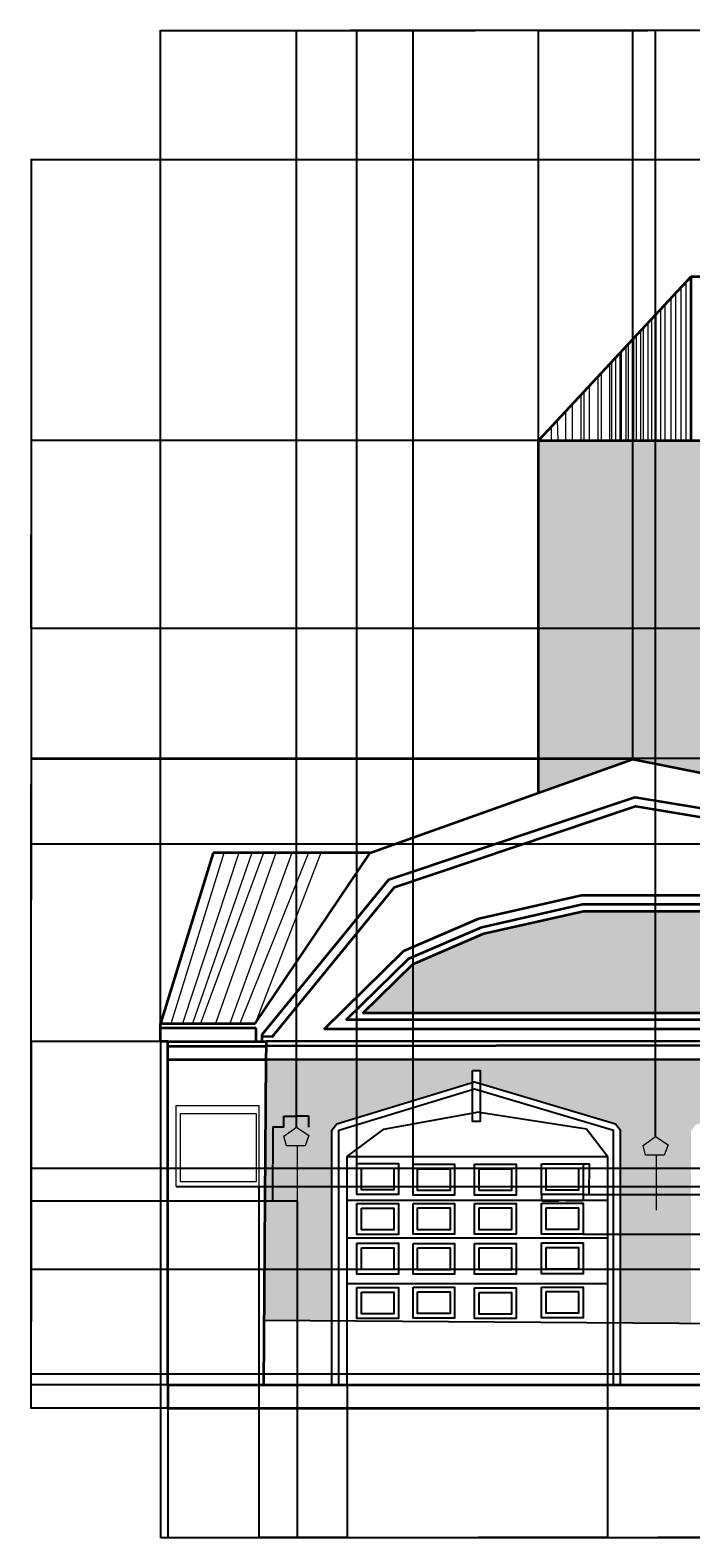
# Model space of a CAD drawing. Units: inches. Extents: x -46 to 1209, y 110 to 778.
# Tile 1 of 5: x -46 to 247, y 110 to 778. Entities that reach past the tile are written whole.
import ezdxf

# ---------------------------------------------------------------- set-up
doc = ezdxf.new("R2010")
doc.units = ezdxf.units.IN
doc.header["$MEASUREMENT"] = 0
for name, color, linetype, lineweight in [('A-ANNO-DIMS', 2, 'Continuous', 18), ('A-DOOR', 3, 'Continuous', 25), ('A-ELEV-BASE', 7, 'Continuous', 35), ('A-GLAZ', 4, 'Continuous', 20), ('A-ROOF', 7, 'Continuous', 35), ('A-ROOF-PATT', 8, 'Continuous', 13), ('A-WALL', 7, 'Continuous', 35), ('A-WALL-PATT', 252, 'Continuous', 13), ('A-WALL-TRIM', 42, 'Continuous', 25), ('E-LITE', 2, 'Continuous', 18)]:
    doc.layers.add(name, color=color, linetype=linetype, lineweight=lineweight)
doc.styles.get("Standard").update_dxf_attribs({"font": 'arial.ttf'})
doc.dimstyles.get("Standard").update_dxf_attribs({"dimtxt": 0.18, "dimasz": 0.18, "dimexe": 0.18, "dimexo": 0.0625, "dimgap": 0.09, "dimtad": 0, "dimtih": 1, "dimtoh": 1, "dimdec": 4, "dimzin": 0, "dimdsep": 46, "dimtxsty": 'Standard', "dimcen": 0.09, "dimadec": 0, "dimazin": 0, "dimtfac": 1, "dimtdec": 4, "dimtofl": 0, "dimtmove": 0, "dimatfit": 3, "dimfxl": 1, "dimtolj": 1, "dimtzin": 0, "dimarcsym": 0})

# ---------------------------------------------------------------- blocks, each defined once
blk = doc.blocks.new('WIN-SMALL-FRAME')
for points in [[(0, 35.97), (36.6, 35.97), (36.6, 0), (0, 0)], [(1.9, 32.4), (35.37, 32.4), (35.37, 2.05), (1.9, 2.05)]]:
    blk.add_lwpolyline(points, close=True)
blk = doc.blocks.new('PANEL-GARAGE-RAISED')
for points in [[(0, 13.64), (18.32, 13.64), (18.32, 0), (0, 0)], [(2, 11.64), (16.32, 11.64), (16.32, 2), (2, 2)]]:
    blk.add_lwpolyline(points, close=True)
blk = doc.blocks.new('KEYSTONE-GARAGE')
blk.add_lwpolyline([(0, 22.61), (3.38, 22.61), (3.38, 0), (0, 0)], close=True)
blk = doc.blocks.new('LIGHT-EXT-GARAGE')
blk.add_line((5.84, 24.47), (5.84, 0))
blk.add_lwpolyline([(5.84, 24.47), (1.13, 24.47), (0, 28.75), (5.52, 32.71), (11.04, 29.03), (9.34, 24.47), (5.84, 24.47)])
blk = doc.blocks.new('*D10')
at = {"layer": 'A-ANNO-DIMS', "color": 0, "lineweight": -2, "transparency": 16777216}
for p, q in [((180.55, 261.88), (180.55, 259.01)), ((198.86, 261.88), (198.86, 259.01)), ((180.73, 259.19), (188.16, 259.19)), ((198.68, 259.19), (191.25, 259.19))]:
    blk.add_line(p, q, dxfattribs=at)
at = {"layer": 'A-ANNO-DIMS', "color": 0, "transparency": 16777216}
for points in [[(180.73, 259.22), (180.73, 259.16), (180.55, 259.19)], [(198.68, 259.22), (198.68, 259.16), (198.86, 259.19)]]:
    blk.add_solid(points, dxfattribs=at)
at = {"layer": 'Defpoints', "color": 0, "transparency": 16777216}
for p in [(180.55, 261.94), (198.86, 261.94), (198.86, 259.19)]:
    blk.add_point(p, dxfattribs=at)
at = {"layer": 'A-ANNO-DIMS', "color": 0, "transparency": 16777216, "insert": (189.71, 259.19), "char_height": 0.18, "attachment_point": 5}
blk.add_mtext('\\A1;GARAGE PANEL 18 TYP.', dxfattribs=at)
blk = doc.blocks.new('*D11')
at = {"layer": 'A-ANNO-DIMS', "color": 0, "lineweight": -2, "transparency": 16777216}
for p, q in [((198.93, 275.58), (201.79, 275.58)), ((201.61, 275.4), (201.61, 268.94)), ((201.61, 262.12), (201.61, 268.58)), ((198.93, 261.94), (201.79, 261.94))]:
    blk.add_line(p, q, dxfattribs=at)
at = {"layer": 'A-ANNO-DIMS', "color": 0, "transparency": 16777216}
for points in [[(201.58, 275.4), (201.64, 275.4), (201.61, 275.58)], [(201.58, 262.12), (201.64, 262.12), (201.61, 261.94)]]:
    blk.add_solid(points, dxfattribs=at)
at = {"layer": 'Defpoints', "color": 0, "transparency": 16777216}
for p in [(198.86, 275.58), (201.61, 275.58), (198.86, 261.94)]:
    blk.add_point(p, dxfattribs=at)
at = {"layer": 'A-ANNO-DIMS', "color": 0, "transparency": 16777216, "insert": (201.61, 268.76), "char_height": 0.18, "attachment_point": 5}
blk.add_mtext('\\A1;14 TYP.', dxfattribs=at)
blk = doc.blocks.new('*D26')
at = {"layer": 'A-ANNO-DIMS', "color": 0, "lineweight": -2, "transparency": 16777216}
for p, q in [((66.52, 291.75), (61.49, 291.75)), ((61.67, 291.57), (61.67, 275.57)), ((61.67, 259.22), (61.67, 275.21)), ((66.52, 259.04), (61.49, 259.04))]:
    blk.add_line(p, q, dxfattribs=at)
at = {"layer": 'A-ANNO-DIMS', "color": 0, "transparency": 16777216}
for points in [[(61.64, 291.57), (61.7, 291.57), (61.67, 291.75)], [(61.64, 259.22), (61.7, 259.22), (61.67, 259.04)]]:
    blk.add_solid(points, dxfattribs=at)
at = {"layer": 'Defpoints', "color": 0, "transparency": 16777216}
for p in [(61.67, 291.75), (66.58, 291.75), (66.58, 259.04)]:
    blk.add_point(p, dxfattribs=at)
at = {"layer": 'A-ANNO-DIMS', "color": 0, "transparency": 16777216, "insert": (61.67, 275.39), "char_height": 0.18, "attachment_point": 5}
blk.add_mtext('\\A1;WALL LIGHT 33 TYP.', dxfattribs=at)
blk = doc.blocks.new('*D27')
at = {"layer": 'A-ANNO-DIMS', "color": 0, "lineweight": -2, "transparency": 16777216}
for p, q in [((66.58, 291.81), (66.58, 296.83)), ((66.76, 296.65), (71.58, 296.65)), ((77.44, 296.65), (72.62, 296.65)), ((77.62, 291.81), (77.62, 296.83))]:
    blk.add_line(p, q, dxfattribs=at)
at = {"layer": 'A-ANNO-DIMS', "color": 0, "transparency": 16777216}
for points in [[(66.76, 296.68), (66.76, 296.62), (66.58, 296.65)], [(77.44, 296.68), (77.44, 296.62), (77.62, 296.65)]]:
    blk.add_solid(points, dxfattribs=at)
at = {"layer": 'Defpoints', "color": 0, "transparency": 16777216}
for p in [(77.62, 296.65), (66.58, 291.75), (77.62, 291.75)]:
    blk.add_point(p, dxfattribs=at)
at = {"layer": 'A-ANNO-DIMS', "color": 0, "transparency": 16777216, "insert": (72.1, 296.65), "char_height": 0.18, "attachment_point": 5}
blk.add_mtext('\\A1;11 TYP.', dxfattribs=at)
blk = doc.blocks.new('*D28')
at = {"layer": 'A-ANNO-DIMS', "color": 0, "lineweight": -2, "transparency": 16777216}
for p, q in [((11.98, 329.67), (11.98, 109.96)), ((1151.8, 167.37), (1151.8, 109.96)), ((12.16, 110.14), (581.44, 110.14)), ((1151.62, 110.14), (582.35, 110.14))]:
    blk.add_line(p, q, dxfattribs=at)
at = {"layer": 'A-ANNO-DIMS', "color": 0, "transparency": 16777216}
for points in [[(12.16, 110.17), (12.16, 110.11), (11.98, 110.14)], [(1151.62, 110.17), (1151.62, 110.11), (1151.8, 110.14)]]:
    blk.add_solid(points, dxfattribs=at)
at = {"layer": 'Defpoints', "color": 0, "transparency": 16777216}
for p in [(11.98, 329.73), (1151.8, 167.44), (1151.8, 110.14)]:
    blk.add_point(p, dxfattribs=at)
at = {"layer": 'A-ANNO-DIMS', "color": 0, "transparency": 16777216, "insert": (581.89, 110.14), "char_height": 0.18, "attachment_point": 5}
blk.add_mtext('\\A1;1139.8', dxfattribs=at)
blk = doc.blocks.new('*D29')
at = {"layer": 'A-ANNO-DIMS', "color": 0, "lineweight": -2, "transparency": 16777216}
for p, q in [((456.52, 720.07), (-45.5, 720.07)), ((-45.32, 719.89), (-45.32, 443.93)), ((-45.32, 167.62), (-45.32, 443.57)), ((15.16, 167.44), (-45.5, 167.44))]:
    blk.add_line(p, q, dxfattribs=at)
at = {"layer": 'A-ANNO-DIMS', "color": 0, "transparency": 16777216}
for points in [[(-45.35, 719.89), (-45.29, 719.89), (-45.32, 720.07)], [(-45.35, 167.62), (-45.29, 167.62), (-45.32, 167.44)]]:
    blk.add_solid(points, dxfattribs=at)
at = {"layer": 'Defpoints', "color": 0, "transparency": 16777216}
for p in [(-45.32, 720.07), (456.58, 720.07), (15.23, 167.44)]:
    blk.add_point(p, dxfattribs=at)
at = {"layer": 'A-ANNO-DIMS', "color": 0, "transparency": 16777216, "insert": (-45.32, 443.75), "char_height": 0.18, "attachment_point": 5}
blk.add_mtext('\\A1;552.6', dxfattribs=at)
blk = doc.blocks.new('*D30')
at = {"layer": 'A-ANNO-DIMS', "color": 0, "lineweight": -2, "transparency": 16777216}
for p, q in [((15.23, 177.67), (15.23, 109.96)), ((94.52, 177.67), (94.52, 109.96)), ((15.41, 110.14), (54.48, 110.14)), ((94.34, 110.14), (55.26, 110.14))]:
    blk.add_line(p, q, dxfattribs=at)
at = {"layer": 'A-ANNO-DIMS', "color": 0, "transparency": 16777216}
for points in [[(15.41, 110.17), (15.41, 110.11), (15.23, 110.14)], [(94.34, 110.17), (94.34, 110.11), (94.52, 110.14)]]:
    blk.add_solid(points, dxfattribs=at)
at = {"layer": 'Defpoints', "color": 0, "transparency": 16777216}
for p in [(15.23, 177.73), (94.52, 177.73), (94.52, 110.14)]:
    blk.add_point(p, dxfattribs=at)
at = {"layer": 'A-ANNO-DIMS', "color": 0, "transparency": 16777216, "insert": (54.87, 110.14), "char_height": 0.18, "attachment_point": 5}
blk.add_mtext('\\A1;79.29', dxfattribs=at)
blk = doc.blocks.new('*D31')
at = {"layer": 'A-ANNO-DIMS', "color": 0, "lineweight": -2, "transparency": 16777216}
for p, q in [((94.52, 177.67), (94.52, 109.96)), ((209.64, 177.67), (209.64, 109.96)), ((94.7, 110.14), (151.62, 110.14)), ((209.46, 110.14), (152.53, 110.14))]:
    blk.add_line(p, q, dxfattribs=at)
at = {"layer": 'A-ANNO-DIMS', "color": 0, "transparency": 16777216}
for points in [[(94.7, 110.17), (94.7, 110.11), (94.52, 110.14)], [(209.46, 110.17), (209.46, 110.11), (209.64, 110.14)]]:
    blk.add_solid(points, dxfattribs=at)
at = {"layer": 'Defpoints', "color": 0, "transparency": 16777216}
for p in [(94.52, 177.73), (209.64, 177.73), (209.64, 110.14)]:
    blk.add_point(p, dxfattribs=at)
at = {"layer": 'A-ANNO-DIMS', "color": 0, "transparency": 16777216, "insert": (152.08, 110.14), "char_height": 0.18, "attachment_point": 5}
blk.add_mtext('\\A1;115.12', dxfattribs=at)
blk = doc.blocks.new('*D32')
at = {"layer": 'A-ANNO-DIMS', "color": 0, "lineweight": -2, "transparency": 16777216}
for p, q in [((209.64, 177.67), (209.64, 109.96)), ((253.32, 177.67), (253.32, 109.96)), ((209.82, 110.14), (231.08, 110.14)), ((253.14, 110.14), (231.88, 110.14))]:
    blk.add_line(p, q, dxfattribs=at)
at = {"layer": 'A-ANNO-DIMS', "color": 0, "transparency": 16777216}
for points in [[(209.82, 110.17), (209.82, 110.11), (209.64, 110.14)], [(253.14, 110.17), (253.14, 110.11), (253.32, 110.14)]]:
    blk.add_solid(points, dxfattribs=at)
at = {"layer": 'Defpoints', "color": 0, "transparency": 16777216}
for p in [(209.64, 177.73), (253.32, 177.73), (253.32, 110.14)]:
    blk.add_point(p, dxfattribs=at)
at = {"layer": 'A-ANNO-DIMS', "color": 0, "transparency": 16777216, "insert": (231.48, 110.14), "char_height": 0.18, "attachment_point": 5}
blk.add_mtext('\\A1;43.68', dxfattribs=at)
blk = doc.blocks.new('*D37')
at = {"layer": 'A-ANNO-DIMS', "color": 0, "lineweight": -2, "transparency": 16777216}
for p, q in [((11.92, 329.73), (-45.5, 329.73)), ((-45.32, 329.55), (-45.32, 253.91)), ((-45.32, 177.91), (-45.32, 253.55)), ((15.16, 177.73), (-45.5, 177.73))]:
    blk.add_line(p, q, dxfattribs=at)
at = {"layer": 'A-ANNO-DIMS', "color": 0, "transparency": 16777216}
for points in [[(-45.35, 329.55), (-45.29, 329.55), (-45.32, 329.73)], [(-45.35, 177.91), (-45.29, 177.91), (-45.32, 177.73)]]:
    blk.add_solid(points, dxfattribs=at)
at = {"layer": 'Defpoints', "color": 0, "transparency": 16777216}
for p in [(-45.32, 329.73), (11.98, 329.73), (15.23, 177.73)]:
    blk.add_point(p, dxfattribs=at)
at = {"layer": 'A-ANNO-DIMS', "color": 0, "transparency": 16777216, "insert": (-45.32, 253.73), "char_height": 0.18, "attachment_point": 5}
blk.add_mtext('\\A1;152', dxfattribs=at)
blk = doc.blocks.new('*D38')
at = {"layer": 'A-ANNO-DIMS', "color": 0, "lineweight": -2, "transparency": 16777216}
for p, q in [((220.83, 454.72), (-45.5, 454.72)), ((-45.32, 454.54), (-45.32, 392.41)), ((-45.32, 329.91), (-45.32, 392.04)), ((11.92, 329.73), (-45.5, 329.73))]:
    blk.add_line(p, q, dxfattribs=at)
at = {"layer": 'A-ANNO-DIMS', "color": 0, "transparency": 16777216}
for points in [[(-45.35, 454.54), (-45.29, 454.54), (-45.32, 454.72)], [(-45.35, 329.91), (-45.29, 329.91), (-45.32, 329.73)]]:
    blk.add_solid(points, dxfattribs=at)
at = {"layer": 'Defpoints', "color": 0, "transparency": 16777216}
for p in [(-45.32, 454.72), (220.89, 454.72), (11.98, 329.73)]:
    blk.add_point(p, dxfattribs=at)
at = {"layer": 'A-ANNO-DIMS', "color": 0, "transparency": 16777216, "insert": (-45.32, 392.23), "char_height": 0.18, "attachment_point": 5}
blk.add_mtext('\\A1;124.99', dxfattribs=at)
blk = doc.blocks.new('*D39')
at = {"layer": 'A-ANNO-DIMS', "color": 0, "lineweight": -2, "transparency": 16777216}
for p, q in [((11.98, 337.79), (11.98, 777.55)), ((12.16, 777.37), (116.04, 777.37)), ((220.71, 777.37), (116.83, 777.37)), ((220.89, 454.78), (220.89, 777.55))]:
    blk.add_line(p, q, dxfattribs=at)
at = {"layer": 'A-ANNO-DIMS', "color": 0, "transparency": 16777216}
for points in [[(12.16, 777.4), (12.16, 777.34), (11.98, 777.37)], [(220.71, 777.4), (220.71, 777.34), (220.89, 777.37)]]:
    blk.add_solid(points, dxfattribs=at)
at = {"layer": 'Defpoints', "color": 0, "transparency": 16777216}
for p in [(220.89, 777.37), (220.89, 454.72), (11.98, 337.73)]:
    blk.add_point(p, dxfattribs=at)
at = {"layer": 'A-ANNO-DIMS', "color": 0, "transparency": 16777216, "insert": (116.44, 777.37), "char_height": 0.18, "attachment_point": 5}
blk.add_mtext('\\A1;208.9', dxfattribs=at)
blk = doc.blocks.new('*D40')
at = {"layer": 'A-ANNO-DIMS', "color": 0, "lineweight": -2, "transparency": 16777216}
for p, q in [((98.84, 275.74), (98.84, 777.55)), ((99.02, 777.37), (110.8, 777.37)), ((123.52, 777.37), (111.73, 777.37)), ((123.7, 275.45), (123.7, 777.55))]:
    blk.add_line(p, q, dxfattribs=at)
at = {"layer": 'A-ANNO-DIMS', "color": 0, "transparency": 16777216}
for points in [[(99.02, 777.4), (99.02, 777.34), (98.84, 777.37)], [(123.52, 777.4), (123.52, 777.34), (123.7, 777.37)]]:
    blk.add_solid(points, dxfattribs=at)
at = {"layer": 'Defpoints', "color": 0, "transparency": 16777216}
for p in [(123.7, 777.37), (98.84, 275.68), (123.7, 275.39)]:
    blk.add_point(p, dxfattribs=at)
at = {"layer": 'A-ANNO-DIMS', "color": 0, "transparency": 16777216, "insert": (111.27, 777.37), "char_height": 0.18, "attachment_point": 5}
blk.add_mtext('\\A1;24.863', dxfattribs=at)
blk = doc.blocks.new('*D41')
at = {"layer": 'A-ANNO-DIMS', "color": 0, "lineweight": -2, "transparency": 16777216}
for p, q in [((198.93, 261.94), (1209.28, 261.94)), ((1209.1, 261.76), (1209.1, 253.4)), ((1209.1, 244.67), (1209.1, 253.04)), ((198.93, 244.49), (1209.28, 244.49))]:
    blk.add_line(p, q, dxfattribs=at)
at = {"layer": 'A-ANNO-DIMS', "color": 0, "transparency": 16777216}
for points in [[(1209.07, 261.76), (1209.13, 261.76), (1209.1, 261.94)], [(1209.07, 244.67), (1209.13, 244.67), (1209.1, 244.49)]]:
    blk.add_solid(points, dxfattribs=at)
at = {"layer": 'Defpoints', "color": 0, "transparency": 16777216}
for p in [(198.86, 261.94), (1209.1, 261.94), (198.86, 244.49)]:
    blk.add_point(p, dxfattribs=at)
at = {"layer": 'A-ANNO-DIMS', "color": 0, "transparency": 16777216, "insert": (1209.1, 253.22), "char_height": 0.18, "attachment_point": 5}
blk.add_mtext('\\A1;17.446', dxfattribs=at)
blk = doc.blocks.new('*D42')
at = {"layer": 'A-ANNO-DIMS', "color": 0, "lineweight": -2, "transparency": 16777216}
for p, q in [((72.1, 291.81), (72.1, 777.55)), ((72.28, 777.37), (151.07, 777.37)), ((230.76, 777.37), (151.98, 777.37)), ((230.94, 287.75), (230.94, 777.55))]:
    blk.add_line(p, q, dxfattribs=at)
at = {"layer": 'A-ANNO-DIMS', "color": 0, "transparency": 16777216}
for points in [[(72.28, 777.4), (72.28, 777.34), (72.1, 777.37)], [(230.76, 777.4), (230.76, 777.34), (230.94, 777.37)]]:
    blk.add_solid(points, dxfattribs=at)
at = {"layer": 'Defpoints', "color": 0, "transparency": 16777216}
for p in [(230.94, 777.37), (72.1, 291.75), (230.94, 287.69)]:
    blk.add_point(p, dxfattribs=at)
at = {"layer": 'A-ANNO-DIMS', "color": 0, "transparency": 16777216, "insert": (151.52, 777.37), "char_height": 0.18, "attachment_point": 5}
blk.add_mtext('\\A1;158.84', dxfattribs=at)
blk = doc.blocks.new('*D43')
at = {"layer": 'A-ANNO-DIMS', "color": 0, "lineweight": -2, "transparency": 16777216}
for p, q in [((55.49, 265.41), (55.49, 109.96)), ((72.42, 258.97), (72.42, 109.96)), ((55.67, 110.14), (63.5, 110.14)), ((72.24, 110.14), (64.41, 110.14))]:
    blk.add_line(p, q, dxfattribs=at)
at = {"layer": 'A-ANNO-DIMS', "color": 0, "transparency": 16777216}
for points in [[(55.67, 110.17), (55.67, 110.11), (55.49, 110.14)], [(72.24, 110.17), (72.24, 110.11), (72.42, 110.14)]]:
    blk.add_solid(points, dxfattribs=at)
at = {"layer": 'Defpoints', "color": 0, "transparency": 16777216}
for p in [(55.49, 265.48), (72.42, 259.04), (72.42, 110.14)]:
    blk.add_point(p, dxfattribs=at)
at = {"layer": 'A-ANNO-DIMS', "color": 0, "transparency": 16777216, "insert": (63.96, 110.14), "char_height": 0.18, "attachment_point": 5}
blk.add_mtext('\\A1;16.934', dxfattribs=at)
blk = doc.blocks.new('*D44')
at = {"layer": 'A-ANNO-DIMS', "color": 0, "lineweight": -2, "transparency": 16777216}
for p, q in [((18.95, 265.48), (1209.28, 265.48)), ((1209.1, 265.3), (1209.1, 221.79)), ((1209.1, 177.91), (1209.1, 221.42)), ((15.29, 177.73), (1209.28, 177.73))]:
    blk.add_line(p, q, dxfattribs=at)
at = {"layer": 'A-ANNO-DIMS', "color": 0, "transparency": 16777216}
for points in [[(1209.07, 265.3), (1209.13, 265.3), (1209.1, 265.48)], [(1209.07, 177.91), (1209.13, 177.91), (1209.1, 177.73)]]:
    blk.add_solid(points, dxfattribs=at)
at = {"layer": 'Defpoints', "color": 0, "transparency": 16777216}
for p in [(18.89, 265.48), (1209.1, 265.48), (15.23, 177.73)]:
    blk.add_point(p, dxfattribs=at)
at = {"layer": 'A-ANNO-DIMS', "color": 0, "transparency": 16777216, "insert": (1209.1, 221.6), "char_height": 0.18, "attachment_point": 5}
blk.add_mtext('\\A1;87.74', dxfattribs=at)
blk = doc.blocks.new('*D45')
at = {"layer": 'A-ANNO-DIMS', "color": 0, "lineweight": -2, "transparency": 16777216}
for p, q in [((72.36, 259.04), (-45.5, 259.04)), ((-45.32, 258.86), (-45.32, 218.57)), ((-45.32, 177.91), (-45.32, 218.2)), ((94.45, 177.73), (-45.5, 177.73))]:
    blk.add_line(p, q, dxfattribs=at)
at = {"layer": 'A-ANNO-DIMS', "color": 0, "transparency": 16777216}
for points in [[(-45.35, 258.86), (-45.29, 258.86), (-45.32, 259.04)], [(-45.35, 177.91), (-45.29, 177.91), (-45.32, 177.73)]]:
    blk.add_solid(points, dxfattribs=at)
at = {"layer": 'Defpoints', "color": 0, "transparency": 16777216}
for p in [(72.42, 259.04), (-45.32, 177.73), (94.52, 177.73)]:
    blk.add_point(p, dxfattribs=at)
at = {"layer": 'A-ANNO-DIMS', "color": 0, "transparency": 16777216, "insert": (-45.32, 218.38), "char_height": 0.18, "attachment_point": 5}
blk.add_mtext('\\A1;81.3', dxfattribs=at)
blk = doc.blocks.new('*D49')
at = {"layer": 'A-ANNO-DIMS', "color": 0, "lineweight": -2, "transparency": 16777216}
for p, q in [((488.59, 273.51), (-45.5, 273.51)), ((-45.32, 273.33), (-45.32, 225.8)), ((-45.32, 177.91), (-45.32, 225.44)), ((488.59, 177.73), (-45.5, 177.73))]:
    blk.add_line(p, q, dxfattribs=at)
at = {"layer": 'A-ANNO-DIMS', "color": 0, "transparency": 16777216}
for points in [[(-45.35, 273.33), (-45.29, 273.33), (-45.32, 273.51)], [(-45.35, 177.91), (-45.29, 177.91), (-45.32, 177.73)]]:
    blk.add_solid(points, dxfattribs=at)
at = {"layer": 'Defpoints', "color": 0, "transparency": 16777216}
for p in [(-45.32, 273.51), (488.65, 273.51), (488.65, 177.73)]:
    blk.add_point(p, dxfattribs=at)
at = {"layer": 'A-ANNO-DIMS', "color": 0, "transparency": 16777216, "insert": (-45.32, 225.62), "char_height": 0.18, "attachment_point": 5}
blk.add_mtext('\\A1;95.78', dxfattribs=at)
blk = doc.blocks.new('*D52')
at = {"layer": 'A-ANNO-DIMS', "color": 0, "lineweight": -2, "transparency": 16777216}
for p, q in [((492.87, 228.83), (-45.5, 228.83)), ((-45.32, 228.65), (-45.32, 205.81)), ((-45.32, 182.61), (-45.32, 205.45)), ((492.87, 182.43), (-45.5, 182.43))]:
    blk.add_line(p, q, dxfattribs=at)
at = {"layer": 'A-ANNO-DIMS', "color": 0, "transparency": 16777216}
for points in [[(-45.35, 228.65), (-45.29, 228.65), (-45.32, 228.83)], [(-45.35, 182.61), (-45.29, 182.61), (-45.32, 182.43)]]:
    blk.add_solid(points, dxfattribs=at)
at = {"layer": 'Defpoints', "color": 0, "transparency": 16777216}
for p in [(-45.32, 228.83), (492.93, 228.83), (492.93, 182.43)]:
    blk.add_point(p, dxfattribs=at)
at = {"layer": 'A-ANNO-DIMS', "color": 0, "transparency": 16777216, "insert": (-45.32, 205.63), "char_height": 0.18, "attachment_point": 5}
blk.add_mtext('\\A1;46.4', dxfattribs=at)
blk = doc.blocks.new('*D60')
at = {"layer": 'A-ANNO-DIMS', "color": 0, "lineweight": -2, "transparency": 16777216}
for p, q in [((11.98, 337.79), (11.98, 777.55)), ((12.16, 777.37), (95.17, 777.37)), ((178.92, 777.37), (95.91, 777.37)), ((179.1, 595.85), (179.1, 777.55))]:
    blk.add_line(p, q, dxfattribs=at)
at = {"layer": 'A-ANNO-DIMS', "color": 0, "transparency": 16777216}
for points in [[(12.16, 777.4), (12.16, 777.34), (11.98, 777.37)], [(178.92, 777.4), (178.92, 777.34), (179.1, 777.37)]]:
    blk.add_solid(points, dxfattribs=at)
at = {"layer": 'Defpoints', "color": 0, "transparency": 16777216}
for p in [(179.1, 777.37), (179.1, 595.79), (11.98, 337.73)]:
    blk.add_point(p, dxfattribs=at)
at = {"layer": 'A-ANNO-DIMS', "color": 0, "transparency": 16777216, "insert": (95.54, 777.37), "char_height": 0.18, "attachment_point": 5}
blk.add_mtext('\\A1;167.1', dxfattribs=at)
blk = doc.blocks.new('*D61')
at = {"layer": 'A-ANNO-DIMS', "color": 0, "lineweight": -2, "transparency": 16777216}
for p, q in [((179.04, 595.79), (-45.5, 595.79)), ((-45.32, 595.61), (-45.32, 554.39)), ((-45.32, 512.81), (-45.32, 554.03)), ((276.7, 512.63), (-45.5, 512.63))]:
    blk.add_line(p, q, dxfattribs=at)
at = {"layer": 'A-ANNO-DIMS', "color": 0, "transparency": 16777216}
for points in [[(-45.35, 595.61), (-45.29, 595.61), (-45.32, 595.79)], [(-45.35, 512.81), (-45.29, 512.81), (-45.32, 512.63)]]:
    blk.add_solid(points, dxfattribs=at)
at = {"layer": 'Defpoints', "color": 0, "transparency": 16777216}
for p in [(179.1, 595.79), (-45.32, 512.63), (276.76, 512.63)]:
    blk.add_point(p, dxfattribs=at)
at = {"layer": 'A-ANNO-DIMS', "color": 0, "transparency": 16777216, "insert": (-45.32, 554.21), "char_height": 0.18, "attachment_point": 5}
blk.add_mtext('\\A1;83.16', dxfattribs=at)
blk = doc.blocks.new('*D62')
at = {"layer": 'A-ANNO-DIMS', "color": 0, "lineweight": -2, "transparency": 16777216}
for p, q in [((179.1, 595.85), (179.1, 777.55)), ((179.28, 777.37), (227.54, 777.37)), ((276.58, 777.37), (228.33, 777.37)), ((276.76, 512.69), (276.76, 777.55))]:
    blk.add_line(p, q, dxfattribs=at)
at = {"layer": 'A-ANNO-DIMS', "color": 0, "transparency": 16777216}
for points in [[(179.28, 777.4), (179.28, 777.34), (179.1, 777.37)], [(276.58, 777.4), (276.58, 777.34), (276.76, 777.37)]]:
    blk.add_solid(points, dxfattribs=at)
at = {"layer": 'Defpoints', "color": 0, "transparency": 16777216}
for p in [(276.76, 777.37), (179.1, 595.79), (276.76, 512.63)]:
    blk.add_point(p, dxfattribs=at)
at = {"layer": 'A-ANNO-DIMS', "color": 0, "transparency": 16777216, "insert": (227.93, 777.37), "char_height": 0.18, "attachment_point": 5}
blk.add_mtext('\\A1;97.66', dxfattribs=at)
blk = doc.blocks.new('*D67')
at = {"layer": 'A-ANNO-DIMS', "color": 0, "lineweight": -2, "transparency": 16777216}
for p, q in [((683.9, 455.08), (-45.5, 455.08)), ((-45.32, 454.9), (-45.32, 436.29)), ((-45.32, 417.31), (-45.32, 435.93)), ((575.86, 417.13), (-45.5, 417.13))]:
    blk.add_line(p, q, dxfattribs=at)
at = {"layer": 'A-ANNO-DIMS', "color": 0, "transparency": 16777216}
for points in [[(-45.35, 454.9), (-45.29, 454.9), (-45.32, 455.08)], [(-45.35, 417.31), (-45.29, 417.31), (-45.32, 417.13)]]:
    blk.add_solid(points, dxfattribs=at)
at = {"layer": 'Defpoints', "color": 0, "transparency": 16777216}
for p in [(-45.32, 455.08), (683.96, 455.08), (575.92, 417.13)]:
    blk.add_point(p, dxfattribs=at)
at = {"layer": 'A-ANNO-DIMS', "color": 0, "transparency": 16777216, "insert": (-45.32, 436.11), "char_height": 0.18, "attachment_point": 5}
blk.add_mtext('\\A1;37.95', dxfattribs=at)

msp = doc.modelspace()

# ---------------------------------------------------------------- hatches: boundary and pattern name
at = {"layer": 'A-WALL-PATT'}
h = msp.add_hatch(dxfattribs=at)
h.set_pattern_fill('AR-CONC', color=256, scale=3)
h.paths.add_polyline_path([(387.8322, 595.7911), (179.1007, 595.7911), (179.1007, 451.7911), (179.1007, 439.7911), (220.892, 454.7186), (313.6366, 436.1845), (387.8322, 376.346)])
h.paths.add_polyline_path([(276.7646, 548.5945), (292.8821, 548.5945), (292.8821, 553.0308), (295.9402, 553.0308), (295.9402, 548.5945), (313.3682, 548.5945), (313.3682, 512.6263), (276.7646, 512.6263)], flags=16)
h.paths.add_polyline_path([(278.6627, 545.0233), (312.1316, 545.0233), (312.1316, 514.6792), (278.6627, 514.6792)], flags=0)
h.paths.add_polyline_path([(326.2691, 548.5945), (341.5129, 548.5945), (341.5129, 553.0308), (344.571, 553.0308), (344.571, 548.5945), (362.8728, 548.5945), (362.8728, 512.6263), (326.2691, 512.6263)], flags=16)
h.paths.add_polyline_path([(328.1673, 545.0233), (361.6362, 545.0233), (361.6362, 514.6792), (328.1673, 514.6792)], flags=0)
h.paths.add_polyline_path([(651.5361, 595.7911), (415.401, 595.7911), (387.8322, 595.7911), (387.8322, 376.346), (409.6414, 342.2631), (651.5361, 342.2631)])
h.paths.add_polyline_path([(470.5081, 534.2042), (467.0793, 534.2042), (467.0793, 554.4029), (483.2058, 554.4029), (483.2058, 549.2024), (518.0634, 549.2024), (518.0634, 557.4852), (520.3257, 557.4852), (520.3257, 564.6435), (523.2165, 564.6435), (523.2165, 557.4852), (525.4788, 557.4852), (525.4788, 549.2024), (567.4184, 549.2024), (567.4184, 554.4029), (579.1691, 554.4029), (579.1691, 534.2042), (575.9249, 534.2042), (575.9249, 428.1662), (580.259, 428.1662), (580.259, 412.8567), (567.4184, 412.8567), (567.4184, 417.1318), (483.8186, 417.1318), (483.8186, 413.5449), (465.7589, 413.5449), (465.7589, 426.3336), (470.5081, 426.3336)], flags=16)
h.paths.add_polyline_path([(483.2375, 532.926), (568.2834, 532.926), (568.2834, 425.5857), (483.2375, 425.5857)], flags=0)
h.paths.add_polyline_path([(431.7717, 578.8147), (431.7717, 585.9699), (440.9467, 585.9699), (440.9467, 578.8147)], flags=16)
h.paths.add_polyline_path([(423.2681, 578.8147), (414.0931, 578.8147), (414.0931, 585.9699), (423.2681, 585.9699)], flags=16)
h.paths.add_polyline_path([(447.8839, 578.8147), (447.8839, 585.9699), (457.0589, 585.9699), (457.0589, 578.8147)], flags=16)
h.paths.add_polyline_path([(406.5964, 578.8147), (397.4214, 578.8147), (397.4214, 585.9699), (406.5964, 585.9699)], flags=16)
h.paths.add_polyline_path([(466.0101, 578.8147), (466.0101, 585.9699), (475.1851, 585.9699), (475.1851, 578.8147)], flags=16)
h.paths.add_polyline_path([(483.6888, 578.8147), (483.6888, 585.9699), (492.8638, 585.9699), (492.8638, 578.8147)], flags=16)
h.paths.add_polyline_path([(504.0528, 578.8147), (504.0528, 585.9699), (513.2278, 585.9699), (513.2278, 578.8147)], flags=16)
h.paths.add_polyline_path([(523.0742, 578.8147), (523.0742, 585.9699), (532.2492, 585.9699), (532.2492, 578.8147)], flags=16)
h.paths.add_polyline_path([(542.3193, 578.8147), (542.3193, 585.9699), (551.4943, 585.9699), (551.4943, 578.8147)], flags=16)
h.paths.add_polyline_path([(559.998, 578.8147), (559.998, 585.9699), (569.1729, 585.9699), (569.1729, 578.8147)], flags=16)
h.paths.add_polyline_path([(580.1382, 578.8147), (580.1382, 585.9699), (589.3132, 585.9699), (589.3132, 578.8147)], flags=16)
h.paths.add_polyline_path([(598.3313, 578.8147), (598.3313, 585.9699), (607.5063, 585.9699), (607.5063, 578.8147)], flags=16)
h.paths.add_polyline_path([(618.2477, 578.8147), (618.2477, 585.9699), (627.4227, 585.9699), (627.4227, 578.8147)], flags=16)
h.paths.add_polyline_path([(636.8215, 578.8147), (636.8215, 585.9699), (645.9965, 585.9699), (645.9965, 578.8147)], flags=16)
h.paths.add_polyline_path([(1151.8016, 595.7911), (651.5361, 595.7911), (651.5361, 342.2631), (939.9139, 342.2631), (1151.8016, 342.2631)])
h.paths.add_polyline_path([(683.9631, 455.0835), (683.9631, 537.4823), (720.8864, 537.4823), (720.8864, 547.6453), (727.8922, 547.6453), (727.8922, 537.4823), (767.8177, 537.4823), (767.8177, 455.0835)], flags=16)
h.paths.add_polyline_path([(688.3115, 459.7865), (688.3115, 529.3012), (764.9847, 529.3012), (764.9847, 459.7865)], flags=0)
h.paths.add_polyline_path([(840.5045, 455.0835), (840.5045, 537.4823), (877.4279, 537.4823), (877.4279, 547.6453), (884.4336, 547.6453), (884.4336, 537.4823), (924.3592, 537.4823), (924.3592, 455.0835)], flags=16)
h.paths.add_polyline_path([(844.853, 459.7865), (844.853, 529.3012), (921.5262, 529.3012), (921.5262, 459.7865)], flags=0)
h.paths.add_polyline_path([(994.2223, 455.0835), (994.2223, 537.4823), (1031.1457, 537.4823), (1031.1457, 547.6453), (1038.1514, 547.6453), (1038.1514, 537.4823), (1078.077, 537.4823), (1078.077, 455.0835)], flags=16)
h.paths.add_polyline_path([(998.5708, 459.7865), (998.5708, 529.3012), (1075.244, 529.3012), (1075.244, 459.7865)], flags=0)
h.paths.add_polyline_path([(1151.8016, 321.9907), (941.4829, 321.9907), (632.1261, 321.9907), (632.1261, 313.1625), (629.6322, 313.1625), (629.6322, 281.6236), (635.9059, 281.6236), (635.9059, 276.2471), (629.6322, 276.2471), (629.6322, 185.3878), (632.1261, 185.3878), (632.1261, 177.7316), (1151.8016, 177.7316)])
h.paths.add_polyline_path([(704.3294, 282.1806), (702.3037, 282.1806), (702.3037, 292.8947), (707.3294, 292.8947), (707.3294, 290.4743), (740.8704, 290.4743), (740.8704, 292.7856), (747.2108, 292.7856), (747.2108, 281.5404), (744.5274, 281.5404), (744.5274, 216.7007), (746.4513, 216.7007), (746.4513, 208.2103), (741.5274, 208.2103), (741.5274, 210.4615), (707.3294, 210.4615), (707.3294, 208.0997), (702.1613, 208.0997), (702.1613, 216.7007), (704.3294, 216.7007)], flags=16)
h.paths.add_polyline_path([(707.3294, 287.4743), (741.5274, 287.4743), (741.5274, 213.4615), (707.3294, 213.4615)], flags=0)
h.paths.add_polyline_path([(859.0635, 282.1806), (859.0635, 292.8947), (864.0892, 292.8947), (864.0892, 290.4743), (897.6301, 290.4743), (897.6301, 292.7856), (903.9705, 292.7856), (903.9705, 281.5404), (901.2871, 281.5404), (901.2871, 216.7007), (903.2111, 216.7007), (903.2111, 208.2103), (898.2871, 208.2103), (898.2871, 210.4615), (864.0892, 210.4615), (864.0892, 208.0997), (858.9211, 208.0997), (858.9211, 216.7007), (861.0892, 216.7007), (861.0892, 282.1806)], flags=16)
h.paths.add_polyline_path([(864.0892, 287.4743), (898.2871, 287.4743), (898.2871, 213.4615), (864.0892, 213.4615)], flags=0)
h.paths.add_polyline_path([(1013.4529, 282.1806), (1013.4529, 292.8947), (1018.4786, 292.8947), (1018.4786, 290.4743), (1052.0195, 290.4743), (1052.0195, 292.7856), (1058.3599, 292.7856), (1058.3599, 281.5404), (1055.6765, 281.5404), (1055.6765, 216.7007), (1057.6005, 216.7007), (1057.6005, 208.2103), (1052.6765, 208.2103), (1052.6765, 210.4615), (1018.4786, 210.4615), (1018.4786, 208.0997), (1013.3105, 208.0997), (1013.3105, 216.7007), (1015.4786, 216.7007), (1015.4786, 282.1806)], flags=16)
h.paths.add_polyline_path([(1018.4786, 287.4743), (1052.6765, 287.4743), (1052.6765, 213.4615), (1018.4786, 213.4615)], flags=0)
h.paths.add_polyline_path([(431.9367, 276.2471), (423.7231, 276.2471), (423.7231, 281.6236), (431.9367, 281.6236), (431.9367, 313.1625), (430.3199, 313.1625), (430.3199, 321.9907), (406.6462, 321.9907), (406.6462, 321.7316), (405.6256, 177.7316), (430.3199, 177.7316), (430.3199, 185.3878), (431.9367, 185.3878)])
h.paths.add_polyline_path([(406.6462, 321.7316), (406.6462, 321.9907), (363.2774, 321.9907), (58.5947, 321.7316), (57.7764, 206.2827), (87.7834, 206.0701), (87.7834, 290.4607), (89.9075, 293.33), (149.9611, 311.663), (149.9611, 316.8909), (153.3383, 316.8909), (153.3383, 311.1504), (213.2336, 293.3362), (215.3783, 290.4607), (215.3783, 205.1657), (246.588, 204.9445), (246.588, 290.0127), (248.7121, 292.882), (308.2509, 311.0579), (308.2509, 316.0122), (311.6281, 316.0122), (311.6281, 310.8556), (372.0381, 292.8882), (374.1829, 290.0127), (374.1829, 204.0402), (405.8105, 203.8161)])
h.paths.add_polyline_path([(333, 359.5), (292.5, 377), (250.5, 387.5), (199, 387.5), (155, 377.5), (123.5, 364), (101.4287, 342.2631), (363.2774, 342.2631)])
h.paths.add_polyline_path([(579.9721, 681.6773), (549.8011, 690.7996), (524.9646, 691.17), (482.8908, 691.7975), (447.0968, 679.2482), (416.3264, 659.1694), (597.1807, 659.1694)])

# ---------------------------------------------------------------- linework, layer by layer
at = {"layer": 'A-DOOR'}
for p, q in [((87.7834, 290.4607), (89.9075, 293.33)), ((87.7834, 177.7316), (87.7834, 290.4607)), ((90.7834, 177.7316), (90.7834, 290.4607)), ((212.3783, 177.7316), (212.3783, 290.4607)), ((213.2336, 293.3362), (215.3783, 290.4607)), ((215.3783, 177.7316), (215.3783, 290.4607)), ((94.5158, 177.7316), (94.5158, 278.7768)), ((94.5158, 278.7768), (209.6378, 278.7768)), ((209.6378, 278.7768), (209.6378, 177.7316)), ((94.5158, 259.4499), (209.6378, 259.4499)), ((94.5158, 242.7645), (209.6378, 242.7645)), ((94.5158, 222.5397), (209.6378, 222.5397))]:
    msp.add_line(p, q, dxfattribs=at)
for points in [[(89.9075, 293.33), (150.7772, 311.9122), (213.2336, 293.3362)], [(90.7834, 290.4607), (150.7884, 308.7789), (212.3783, 290.4607)], [(94.5158, 278.7768), (110.7951, 290.9733), (152.0768, 298.4065)], [(209.6378, 278.7768), (200.3217, 290.9733), (152.0768, 298.4065)]]:
    msp.add_lwpolyline(points, dxfattribs=at)
at = {"layer": 'A-ELEV-BASE'}
for p, q in [((15.2259, 177.7316), (1151.8016, 177.7316)), ((15.2259, 177.7316), (15.2259, 167.435)), ((57.5741, 177.7316), (405.6256, 177.7316)), ((15.2259, 167.435), (1151.8016, 167.435))]:
    msp.add_line(p, q, dxfattribs=at)
at = {"layer": 'A-ROOF'}
for p, q in [((246.5295, 668.3019), (179.1007, 595.7911)), ((366.7938, 668.3019), (246.5295, 668.3019)), ((246.5295, 668.3019), (246.5295, 595.7911)), ((35.2829, 413.2214), (11.9842, 337.7316)), ((104.7154, 413.2214), (35.2829, 413.2214)), ((11.9842, 335.7316), (11.9842, 337.7316)), ((11.9842, 337.7316), (53.8945, 337.7316)), ((11.9842, 329.7316), (11.9842, 335.7316)), ((11.9842, 335.7316), (54.0751, 335.7316)), ((54.0751, 335.7316), (54.0751, 329.7316)), ((15.2259, 329.7316), (11.9842, 329.7316)), ((15.2259, 327.7316), (15.2259, 329.7316)), ((15.2259, 329.7316), (58.6514, 329.7316)), ((15.2259, 321.7316), (15.2259, 327.7316)), ((15.2259, 327.7316), (58.6372, 327.7316)), ((54.0751, 332.7316), (54.0751, 329.7316)), ((54.0751, 329.7316), (56.9823, 329.7316)), ((56.9823, 332.0701), (56.9823, 332.8507)), ((61.2975, 331.811), (56.9823, 331.9406)), ((56.9823, 329.7316), (56.9823, 331.811)), ((58.6372, 327.7316), (58.5947, 321.7316)), ((58.6514, 329.7316), (58.6372, 327.7316)), ((363.2632, 327.9907), (58.6372, 327.7316)), ((363.2774, 329.9907), (58.6514, 329.7316)), ((58.5947, 321.7316), (363.2774, 321.9907))]:
    msp.add_line(p, q, dxfattribs=at)
for points in [[(53.8945, 337.7316), (104.7154, 413.2214), (220.892, 454.7186), (313.6366, 436.1845), (387.8322, 376.346), (415.401, 333.2621)], [(56.9823, 332.8507), (113.0259, 401.4848), (221.8022, 437.979), (307.5529, 423.6986), (376.6298, 371.3374), (406.7029, 332.2401)], [(61.2975, 331.811), (115.3935, 398.06), (222.1289, 433.8695), (305.9227, 419.915), (373.7332, 368.5138), (400.1222, 331.7916)], [(56.9823, 331.811), (56.9823, 332.0701)]]:
    msp.add_lwpolyline(points, dxfattribs=at)
for points in [[(84.345, 335.2631), (119.5289, 369.9139), (152.8278, 384.1848), (198.2146, 394.5), (251.3617, 394.5), (294.7521, 383.6524), (336.1293, 365.7734), (389.722, 335.2631)], [(94.1071, 339.2631), (121.7981, 366.5345), (154.0691, 380.3649), (198.6634, 390.5), (250.8693, 390.5), (293.4652, 379.851), (334.3411, 362.1886), (374.6108, 339.2631)], [(101.4287, 342.2631), (123.5, 364), (155, 377.5), (199, 387.5), (250.5, 387.5), (292.5, 377), (333, 359.5), (363.2774, 342.2631)]]:
    msp.add_lwpolyline(points, close=True, dxfattribs=at)
at = {"layer": 'A-ROOF-PATT'}
for p, q in [((239.7489, 661.0102), (239.7489, 595.7911)), ((242.1207, 663.5608), (242.1207, 595.7911)), ((244.2611, 665.8625), (244.2611, 595.7911)), ((234.9665, 655.8674), (234.9665, 595.7911)), ((237.7285, 658.8376), (237.7285, 595.7911)), ((227.5036, 647.842), (227.5036, 595.7911)), ((229.0946, 649.553), (229.0946, 595.7911)), ((231.0672, 651.6743), (231.0672, 595.7911)), ((233.1633, 653.9283), (233.1633, 595.7911)), ((221.2428, 641.1094), (221.2428, 595.7911)), ((222.2866, 642.2318), (222.2866, 595.7911)), ((224.299, 644.3959), (224.299, 595.7911)), ((225.4515, 645.6353), (225.4515, 595.7911)), ((215.0847, 634.4872), (215.0847, 595.7911)), ((215.7796, 635.2345), (215.7796, 595.7911)), ((217.7175, 637.3185), (217.7175, 595.7911)), ((218.7771, 638.4578), (218.7771, 595.7911)), ((210.5772, 629.6399), (210.5772, 595.7911)), ((211.4634, 630.5929), (211.4634, 595.7911)), ((213.2814, 632.5479), (213.2814, 595.7911)), ((205.4385, 624.1139), (205.4385, 595.7911)), ((206.9006, 625.6862), (206.9006, 595.7911)), ((197.868, 615.9729), (197.868, 595.7911)), ((199.1566, 617.3586), (199.1566, 595.7911)), ((201.5833, 619.9682), (201.5833, 595.7911)), ((191.1134, 608.7092), (191.1134, 595.7911)), ((194.0828, 611.9024), (194.0828, 595.7911)), ((184.7349, 601.85), (184.7349, 595.7911)), ((187.4704, 604.7916), (187.6864, 595.7911)), ((16.5979, 337.7316), (40.173, 413.2214)), ((46.6317, 413.2214), (21.6403, 337.7316)), ((52.382, 413.2214), (26.0635, 337.7316)), ((57.4688, 413.2214), (29.6021, 337.7316)), ((62.9978, 413.2214), (36.237, 337.7316)), ((69.9992, 413.2214), (42.6508, 337.7316)), ((77.3735, 413.2214), (47.0741, 337.7316)), ((82.9026, 413.2214), (53.8945, 337.7316))]:
    msp.add_line(p, q, dxfattribs=at)
at = {"layer": 'A-WALL'}
for p, q in [((179.1007, 451.7911), (179.1007, 595.7911)), ((179.1007, 595.7911), (415.401, 595.7911)), ((179.1007, 439.7911), (179.1007, 451.7911)), ((15.2259, 177.7316), (15.2259, 321.7316)), ((15.2259, 321.7316), (58.5947, 321.7316)), ((58.5947, 321.7316), (57.5741, 177.7316))]:
    msp.add_line(p, q, dxfattribs=at)
at = {"layer": 'A-WALL-TRIM'}
msp.add_line((57.7764, 206.2827), (405.8105, 203.8161), dxfattribs=at)

# ---------------------------------------------------------------- block references
at = {"layer": 'A-DOOR'}
for name, p in [('KEYSTONE-GARAGE', (149.9611, 294.2819)), ('PANEL-GARAGE-RAISED', (98.8377, 262.0405)), ('PANEL-GARAGE-RAISED', (123.7012, 261.7525)), ('PANEL-GARAGE-RAISED', (150.8968, 261.7525)), ('PANEL-GARAGE-RAISED', (180.5475, 261.9412)), ('PANEL-GARAGE-RAISED', (98.8377, 244.3248)), ('PANEL-GARAGE-RAISED', (123.7012, 244.3697)), ('PANEL-GARAGE-RAISED', (150.8968, 244.3697)), ('PANEL-GARAGE-RAISED', (180.5475, 244.4949)), ('PANEL-GARAGE-RAISED', (98.8377, 226.7501)), ('PANEL-GARAGE-RAISED', (180.5475, 226.9259)), ('PANEL-GARAGE-RAISED', (123.7012, 226.6796)), ('PANEL-GARAGE-RAISED', (150.8968, 226.6796)), ('PANEL-GARAGE-RAISED', (98.8377, 207.1307)), ('PANEL-GARAGE-RAISED', (123.7012, 207.2931)), ('PANEL-GARAGE-RAISED', (150.8968, 207.0245)), ('PANEL-GARAGE-RAISED', (180.5475, 207.3838))]:
    msp.add_blockref(name, p, dxfattribs=at)
at = {"layer": 'A-GLAZ'}
msp.add_blockref('WIN-SMALL-FRAME', (18.8869, 265.4762), dxfattribs=at)
at = {"layer": 'E-LITE'}
for p in [(66.5801, 259.0357), (225.4201, 254.9758)]:
    msp.add_blockref('LIGHT-EXT-GARAGE', p, dxfattribs=at)

# ---------------------------------------------------------------- dimensions: what is measured, and where the dimension line sits
at = {"layer": 'A-ANNO-DIMS'}
for base, p1, p2, override, picture, middle in [((220.892, 777.3699), (11.9842, 337.7316), (220.892, 454.7186), {"dimdec": 1, "dimlfac": 1, "dimrnd": 0, "dimzin": 0, "dimdsep": 46, "dimlunit": 2}, '*D39', (116.4381, 777.3699)), ((179.1007, 777.3699), (11.9842, 337.7316), (179.1007, 595.7911), {"dimdec": 1, "dimlfac": 1, "dimrnd": 0, "dimzin": 0, "dimdsep": 46, "dimlunit": 2}, '*D60', (95.5425, 777.3699)), ((230.9419, 777.3699), (72.1018, 291.7477), (230.9419, 287.6879), {"dimdec": 2, "dimlfac": 1, "dimrnd": 0, "dimzin": 0, "dimdsep": 46, "dimlunit": 2}, '*D42', (151.5219, 777.3699)), ((123.70117, 777.36987), (98.8377, 275.67912), (123.70117, 275.39115), {"dimdec": 3, "dimlfac": 1, "dimrnd": 0, "dimzin": 0, "dimdsep": 46, "dimlunit": 2}, '*D40', (111.26944, 777.36987)), ((276.7646, 777.3699), (179.1007, 595.7911), (276.7646, 512.6263), {"dimdec": 2, "dimlfac": 1, "dimrnd": 0, "dimzin": 0, "dimdsep": 46, "dimlunit": 2}, '*D62', (227.9326, 777.3699)), ((1151.8016, 110.135), (11.9842, 329.7316), (1151.8016, 167.435), {"dimdec": 1, "dimlfac": 1, "dimrnd": 0, "dimzin": 0, "dimdsep": 46, "dimlunit": 2}, '*D28', (581.8929, 110.135)), ((72.4246, 110.135), (55.4905, 265.4762), (72.4246, 259.0357), {"dimdec": 3, "dimlfac": 1, "dimrnd": 0, "dimzin": 0, "dimdsep": 46, "dimlunit": 2}, '*D43', (63.9575, 110.135)), ((94.5158, 110.135), (15.2259, 177.7316), (94.5158, 177.7316), {"dimdec": 2, "dimlfac": 1, "dimrnd": 0, "dimzin": 0, "dimdsep": 46, "dimlunit": 2}, '*D30', (54.8708, 110.135)), ((209.6378, 110.135), (94.5158, 177.7316), (209.6378, 177.7316), {"dimdec": 2, "dimlfac": 1, "dimrnd": 0, "dimzin": 0, "dimdsep": 46, "dimlunit": 2}, '*D31', (152.0768, 110.135)), ((253.3203, 110.135), (209.6378, 177.7316), (253.3203, 177.7316), {"dimdec": 2, "dimlfac": 1, "dimrnd": 0, "dimzin": 0, "dimdsep": 46, "dimlunit": 2}, '*D32', (231.4791, 110.135))]:
    dim = msp.add_linear_dim(base=base, p1=p1, p2=p2, dimstyle='Standard', override=override, dxfattribs=at)
    dim.commit()
    dim.dimension.update_dxf_attribs({"geometry": picture, "text_midpoint": middle})
for base, p1, p2, override, picture, middle in [((-45.3158, 720.0699), (15.2259, 167.435), (456.5847, 720.0699), {"dimdec": 1, "dimlfac": 1, "dimrnd": 0, "dimzin": 0, "dimdsep": 46, "dimlunit": 2}, '*D29', (-45.3158, 443.7524)), ((-45.3158, 512.6263), (179.1007, 595.7911), (276.7646, 512.6263), {"dimdec": 2, "dimlfac": 1, "dimrnd": 0, "dimzin": 0, "dimdsep": 46, "dimlunit": 2}, '*D61', (-45.3158, 554.2087)), ((-45.3158, 454.7186), (11.9842, 329.7316), (220.892, 454.7186), {"dimdec": 2, "dimlfac": 1, "dimrnd": 0, "dimzin": 0, "dimdsep": 46, "dimlunit": 2}, '*D38', (-45.3158, 392.2251)), ((-45.3158, 455.0835), (575.9249, 417.1318), (683.9631, 455.0835), {"dimdec": 2, "dimlfac": 1, "dimrnd": 0, "dimzin": 0, "dimdsep": 46, "dimlunit": 2}, '*D67', (-45.3158, 436.1076)), ((-45.3158, 329.7316), (15.2259, 177.7316), (11.9842, 329.7316), {"dimdec": 0, "dimlfac": 1, "dimrnd": 0, "dimzin": 0, "dimdsep": 46, "dimlunit": 2}, '*D37', (-45.3158, 253.7316)), ((-45.3158, 273.5127), (488.6503, 177.7316), (488.6503, 273.5127), {"dimdec": 2, "dimlfac": 1, "dimrnd": 0, "dimzin": 0, "dimdsep": 46, "dimlunit": 2}, '*D49', (-45.3158, 225.6222)), ((1209.1016, 265.4762), (15.2259, 177.7316), (18.8869, 265.4762), {"dimdec": 2, "dimlfac": 1, "dimrnd": 0, "dimzin": 0, "dimdsep": 46, "dimlunit": 2}, '*D44', (1209.1016, 221.6039)), ((1209.1016, 261.9412), (198.8637, 244.4949), (198.8637, 261.9412), {"dimdec": 3, "dimlfac": 1, "dimrnd": 0, "dimzin": 0, "dimdsep": 46, "dimlunit": 2}, '*D41', (1209.1016, 253.218)), ((-45.3158, 177.7316), (72.4246, 259.0357), (94.5158, 177.7316), {"dimdec": 1, "dimlfac": 1, "dimrnd": 0, "dimzin": 0, "dimdsep": 46, "dimlunit": 2}, '*D45', (-45.3158, 218.3837)), ((-45.3158, 228.8283), (492.9346, 182.4306), (492.9346, 228.8283), {"dimdec": 1, "dimlfac": 1, "dimrnd": 0, "dimzin": 0, "dimdsep": 46, "dimlunit": 2}, '*D52', (-45.3158, 205.6294))]:
    dim = msp.add_linear_dim(base=base, p1=p1, p2=p2, angle=90, dimstyle='Standard', override=override, dxfattribs=at)
    dim.commit()
    dim.dimension.update_dxf_attribs({"geometry": picture, "text_midpoint": middle})
for base, p1, p2, text, picture, middle in [((77.6236, 296.6546), (66.5801, 291.7477), (77.6236, 291.7477), '<> TYP.', '*D27', (72.1018, 296.6546)), ((198.8637, 259.1938), (180.5475, 261.9412), (198.8637, 261.9412), 'GARAGE PANEL <> TYP.', '*D10', (189.7056, 259.1938))]:
    dim = msp.add_linear_dim(base=base, p1=p1, p2=p2, text=text, dimstyle='Standard', override={"dimdec": 0, "dimlfac": 1, "dimrnd": 0, "dimzin": 0, "dimdsep": 46, "dimlunit": 2}, dxfattribs=at)
    dim.commit()
    dim.dimension.update_dxf_attribs({"geometry": picture, "text_midpoint": middle})
for base, p1, p2, text, picture, middle in [((61.6733, 291.7477), (66.5801, 259.0357), (66.5801, 291.7477), 'WALL LIGHT <> TYP.', '*D26', (61.6733, 275.3917)), ((201.6111, 275.5799), (198.8637, 261.9412), (198.8637, 275.5799), '<> TYP.', '*D11', (201.6111, 268.7605))]:
    dim = msp.add_linear_dim(base=base, p1=p1, p2=p2, angle=90, text=text, dimstyle='Standard', override={"dimdec": 0, "dimlfac": 1, "dimrnd": 0, "dimzin": 0, "dimdsep": 46, "dimlunit": 2}, dxfattribs=at)
    dim.commit()
    dim.dimension.update_dxf_attribs({"geometry": picture, "text_midpoint": middle})

doc.saveas('drawing.dxf')
